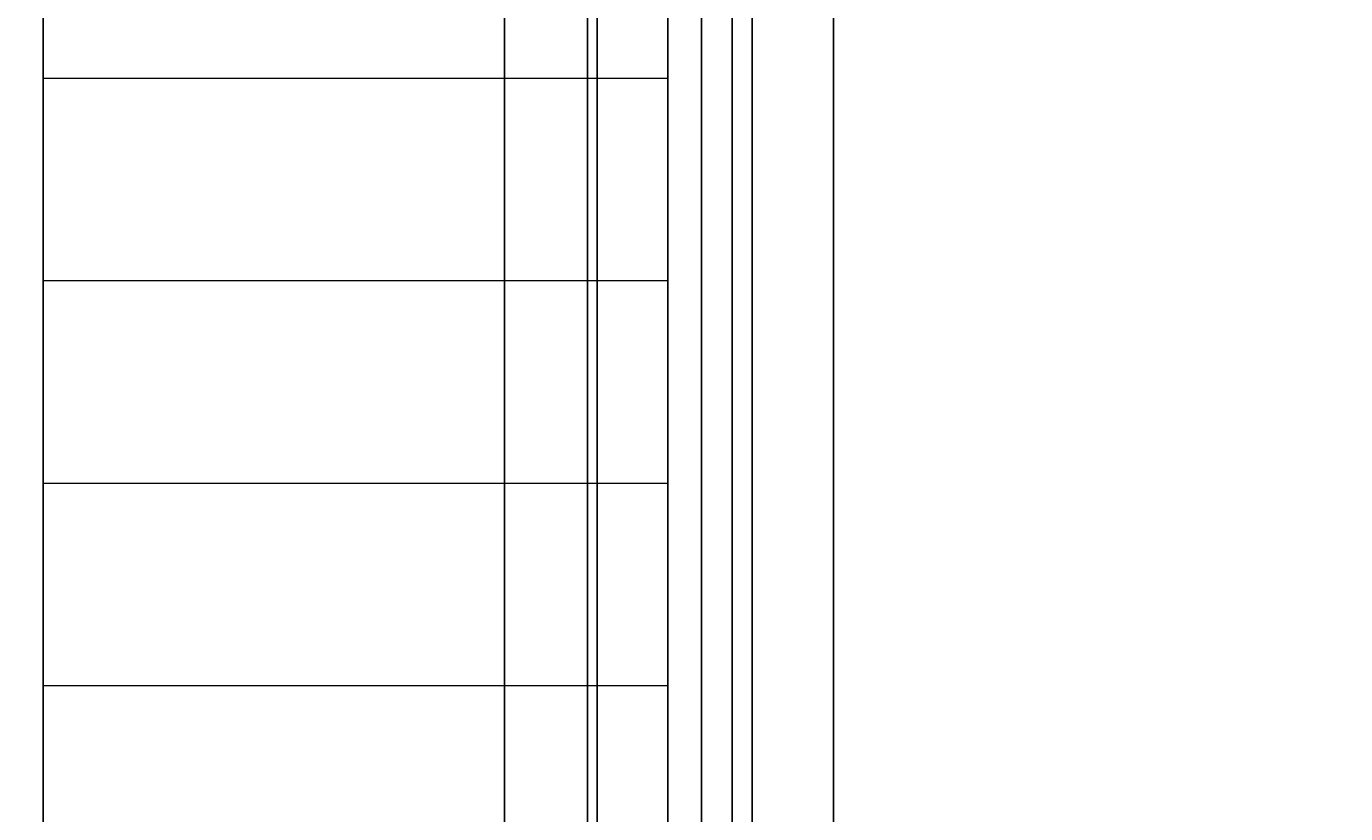
# Model space of a CAD drawing. Units: inches. Extents: x -6 to 289, y -8 to 323.
# Tile 60 of 107: x 147 to 186, y 182 to 206. Entities that reach past the tile are written whole.
import ezdxf

# ---------------------------------------------------------------- set-up
doc = ezdxf.new("R2010")
doc.units = ezdxf.units.IN
doc.header["$MEASUREMENT"] = 0
for name, color, linetype, lineweight in [('A-ANNO-DIMS', 2, 'Continuous', 18), ('A-ELEV-PATT', 8, 'Continuous', 13), ('A-GLAZ', 4, 'Continuous', 25)]:
    doc.layers.add(name, color=color, linetype=linetype, lineweight=lineweight)
doc.styles.get("Standard").update_dxf_attribs({"font": 'arial.ttf'})
doc.dimstyles.get("Standard").update_dxf_attribs({"dimtxt": 0.18, "dimasz": 0.18, "dimexe": 0.18, "dimexo": 0.0625, "dimgap": 0.09, "dimtad": 0, "dimtih": 1, "dimtoh": 1, "dimdec": 4, "dimzin": 0, "dimdsep": 46, "dimtxsty": 'Standard', "dimcen": 0.09, "dimadec": 0, "dimazin": 0, "dimtfac": 1, "dimtdec": 4, "dimtofl": 0, "dimtmove": 0, "dimatfit": 3, "dimfxl": 1, "dimtolj": 1, "dimtzin": 0, "dimarcsym": 0})

# ---------------------------------------------------------------- blocks, each defined once
blk = doc.blocks.new('*U4')
for p, q in [((21, 1.5), (21, 46.5)), ((40.5, 46.5), (40.5, 1.5))]:
    blk.add_line(p, q)
blk.add_lwpolyline([(0, 0), (0, 48), (42, 48), (42, 0)], close=True)
blk.add_lwpolyline([(21, 45.5), (39.5, 45.5), (39.5, 2.5), (21, 2.5)])
blk = doc.blocks.new('*D25')
at = {"layer": 'A-ANNO-DIMS', "color": 0, "lineweight": -2, "transparency": 16777216}
for p, q in [((126.946, 226.654), (288.653, 226.654)), ((288.473, 226.474), (288.473, 202.836)), ((288.473, 178.834), (288.473, 202.472)), ((126.946, 178.654), (288.653, 178.654))]:
    blk.add_line(p, q, dxfattribs=at)
at = {"layer": 'A-ANNO-DIMS', "color": 0, "transparency": 16777216}
for points in [[(288.443, 226.474), (288.503, 226.474), (288.473, 226.654)], [(288.443, 178.834), (288.503, 178.834), (288.473, 178.654)]]:
    blk.add_solid(points, dxfattribs=at)
at = {"layer": 'Defpoints', "color": 0, "transparency": 16777216}
for p in [(126.883, 226.654), (288.473, 226.654), (126.883, 178.654)]:
    blk.add_point(p, dxfattribs=at)
at = {"layer": 'A-ANNO-DIMS', "color": 0, "transparency": 16777216, "insert": (288.473, 202.654), "char_height": 0.18, "attachment_point": 5}
blk.add_mtext('\\A1;48', dxfattribs=at)
blk = doc.blocks.new('*D37')
at = {"layer": 'A-ANNO-DIMS', "color": 0, "lineweight": -2, "transparency": 16777216}
for p, q in [((166.446, 224.154), (288.653, 224.154)), ((288.473, 223.974), (288.473, 202.836)), ((288.473, 181.334), (288.473, 202.472)), ((166.446, 181.154), (288.653, 181.154))]:
    blk.add_line(p, q, dxfattribs=at)
at = {"layer": 'A-ANNO-DIMS', "color": 0, "transparency": 16777216}
for points in [[(288.443, 223.974), (288.503, 223.974), (288.473, 224.154)], [(288.443, 181.334), (288.503, 181.334), (288.473, 181.154)]]:
    blk.add_solid(points, dxfattribs=at)
at = {"layer": 'Defpoints', "color": 0, "transparency": 16777216}
for p in [(166.383, 224.154), (288.473, 224.154), (166.383, 181.154)]:
    blk.add_point(p, dxfattribs=at)
at = {"layer": 'A-ANNO-DIMS', "color": 0, "transparency": 16777216, "insert": (288.473, 202.654), "char_height": 0.18, "attachment_point": 5}
blk.add_mtext('\\A1;43', dxfattribs=at)
blk = doc.blocks.new('*D76')
at = {"layer": 'A-ANNO-DIMS', "color": 0, "lineweight": -2, "transparency": 16777216}
for p, q in [((142.296, 51.148), (142.296, 322.969)), ((164.296, 51.148), (164.296, 322.969)), ((142.476, 322.789), (153.076, 322.789)), ((164.116, 322.789), (153.516, 322.789))]:
    blk.add_line(p, q, dxfattribs=at)
at = {"layer": 'A-ANNO-DIMS', "color": 0, "transparency": 16777216}
for points in [[(142.476, 322.819), (142.476, 322.759), (142.296, 322.789)], [(164.116, 322.819), (164.116, 322.759), (164.296, 322.789)]]:
    blk.add_solid(points, dxfattribs=at)
at = {"layer": 'Defpoints', "color": 0, "transparency": 16777216}
for p in [(164.296, 322.789), (142.296, 51.085), (164.296, 51.085)]:
    blk.add_point(p, dxfattribs=at)
at = {"layer": 'A-ANNO-DIMS', "color": 0, "transparency": 16777216, "insert": (153.296, 322.789), "char_height": 0.18, "attachment_point": 5}
blk.add_mtext('\\A1;22', dxfattribs=at)
blk = doc.blocks.new('*D77')
at = {"layer": 'A-ANNO-DIMS', "color": 0, "lineweight": -2, "transparency": 16777216}
for p, q in [((164.296, 51.148), (164.296, 322.969)), ((168.296, 51.148), (168.296, 322.969)), ((164.476, 322.789), (166.144, 322.789)), ((168.116, 322.789), (166.448, 322.789))]:
    blk.add_line(p, q, dxfattribs=at)
at = {"layer": 'A-ANNO-DIMS', "color": 0, "transparency": 16777216}
for points in [[(164.476, 322.819), (164.476, 322.759), (164.296, 322.789)], [(168.116, 322.819), (168.116, 322.759), (168.296, 322.789)]]:
    blk.add_solid(points, dxfattribs=at)
at = {"layer": 'Defpoints', "color": 0, "transparency": 16777216}
for p in [(168.296, 322.789), (164.296, 51.085), (168.296, 51.085)]:
    blk.add_point(p, dxfattribs=at)
at = {"layer": 'A-ANNO-DIMS', "color": 0, "transparency": 16777216, "insert": (166.296, 322.789), "char_height": 0.18, "attachment_point": 5}
blk.add_mtext('\\A1;4', dxfattribs=at)
blk = doc.blocks.new('*D78')
at = {"layer": 'A-ANNO-DIMS', "color": 0, "lineweight": -2, "transparency": 16777216}
for p, q in [((168.296, 51.148), (168.296, 322.969)), ((171.296, 51.148), (171.296, 322.969)), ((168.476, 322.789), (169.647, 322.789)), ((171.116, 322.789), (169.945, 322.789))]:
    blk.add_line(p, q, dxfattribs=at)
at = {"layer": 'A-ANNO-DIMS', "color": 0, "transparency": 16777216}
for points in [[(168.476, 322.819), (168.476, 322.759), (168.296, 322.789)], [(171.116, 322.819), (171.116, 322.759), (171.296, 322.789)]]:
    blk.add_solid(points, dxfattribs=at)
at = {"layer": 'Defpoints', "color": 0, "transparency": 16777216}
for p in [(171.296, 322.789), (168.296, 51.085), (171.296, 51.085)]:
    blk.add_point(p, dxfattribs=at)
at = {"layer": 'A-ANNO-DIMS', "color": 0, "transparency": 16777216, "insert": (169.796, 322.789), "char_height": 0.18, "attachment_point": 5}
blk.add_mtext('\\A1;3', dxfattribs=at)
blk = doc.blocks.new('*D79')
at = {"layer": 'A-ANNO-DIMS', "color": 0, "lineweight": -2, "transparency": 16777216}
for p, q in [((171.296, 118.033), (171.296, 322.969)), ((188.292, 116.842), (188.292, 322.969)), ((171.476, 322.789), (179.339, 322.789)), ((188.112, 322.789), (180.249, 322.789))]:
    blk.add_line(p, q, dxfattribs=at)
at = {"layer": 'A-ANNO-DIMS', "color": 0, "transparency": 16777216}
for points in [[(171.476, 322.819), (171.476, 322.759), (171.296, 322.789)], [(188.112, 322.819), (188.112, 322.759), (188.292, 322.789)]]:
    blk.add_solid(points, dxfattribs=at)
at = {"layer": 'Defpoints', "color": 0, "transparency": 16777216}
for p in [(188.292, 322.789), (171.296, 117.971), (188.292, 116.779)]:
    blk.add_point(p, dxfattribs=at)
at = {"layer": 'A-ANNO-DIMS', "color": 0, "transparency": 16777216, "insert": (179.794, 322.789), "char_height": 0.18, "attachment_point": 5}
blk.add_mtext('\\A1;16.996', dxfattribs=at)
blk = doc.blocks.new('*D94')
at = {"layer": 'A-ANNO-DIMS', "color": 0, "lineweight": -2, "transparency": 16777216}
for p, q in [((118.164, 159.411), (118.164, 322.969)), ((161.552, 159.411), (161.552, 322.969)), ((118.344, 322.789), (139.46, 322.789)), ((161.372, 322.789), (140.256, 322.789))]:
    blk.add_line(p, q, dxfattribs=at)
at = {"layer": 'A-ANNO-DIMS', "color": 0, "transparency": 16777216}
for points in [[(118.344, 322.819), (118.344, 322.759), (118.164, 322.789)], [(161.372, 322.819), (161.372, 322.759), (161.552, 322.789)]]:
    blk.add_solid(points, dxfattribs=at)
at = {"layer": 'Defpoints', "color": 0, "transparency": 16777216}
for p in [(161.552, 322.789), (118.164, 159.348), (161.552, 159.348)]:
    blk.add_point(p, dxfattribs=at)
at = {"layer": 'A-ANNO-DIMS', "color": 0, "transparency": 16777216, "insert": (139.858, 322.789), "char_height": 0.18, "attachment_point": 5}
blk.add_mtext('\\A1;43.39', dxfattribs=at)
blk = doc.blocks.new('*D95')
at = {"layer": 'A-ANNO-DIMS', "color": 0, "lineweight": -2, "transparency": 16777216}
for p, q in [((161.552, 159.411), (161.552, 322.969)), ((164.004, 159.411), (164.004, 322.969)), ((161.732, 322.789), (162.452, 322.789)), ((163.824, 322.789), (163.104, 322.789))]:
    blk.add_line(p, q, dxfattribs=at)
at = {"layer": 'A-ANNO-DIMS', "color": 0, "transparency": 16777216}
for points in [[(161.732, 322.819), (161.732, 322.759), (161.552, 322.789)], [(163.824, 322.819), (163.824, 322.759), (164.004, 322.789)]]:
    blk.add_solid(points, dxfattribs=at)
at = {"layer": 'Defpoints', "color": 0, "transparency": 16777216}
for p in [(164.004, 322.789), (161.552, 159.348), (164.004, 159.348)]:
    blk.add_point(p, dxfattribs=at)
at = {"layer": 'A-ANNO-DIMS', "color": 0, "transparency": 16777216, "insert": (162.778, 322.789), "char_height": 0.18, "attachment_point": 5}
blk.add_mtext('\\A1;2.45', dxfattribs=at)
blk = doc.blocks.new('*D96')
at = {"layer": 'A-ANNO-DIMS', "color": 0, "lineweight": -2, "transparency": 16777216}
for p, q in [((164.004, 159.411), (164.004, 322.969)), ((200.616, 159.411), (200.616, 322.969)), ((164.184, 322.789), (181.934, 322.789)), ((200.436, 322.789), (182.686, 322.789))]:
    blk.add_line(p, q, dxfattribs=at)
at = {"layer": 'A-ANNO-DIMS', "color": 0, "transparency": 16777216}
for points in [[(164.184, 322.819), (164.184, 322.759), (164.004, 322.789)], [(200.436, 322.819), (200.436, 322.759), (200.616, 322.789)]]:
    blk.add_solid(points, dxfattribs=at)
at = {"layer": 'Defpoints', "color": 0, "transparency": 16777216}
for p in [(200.616, 322.789), (164.004, 159.348), (200.616, 159.348)]:
    blk.add_point(p, dxfattribs=at)
at = {"layer": 'A-ANNO-DIMS', "color": 0, "transparency": 16777216, "insert": (182.31, 322.789), "char_height": 0.18, "attachment_point": 5}
blk.add_mtext('\\A1;36.61', dxfattribs=at)

msp = doc.modelspace()

# ---------------------------------------------------------------- hatches: boundary and pattern name
at = {"layer": 'A-ELEV-PATT'}
h = msp.add_hatch(dxfattribs=at)
h.set_pattern_fill('_USER', color=256, scale=6, pattern_type=0)
h.set_pattern_definition([(0, (0, 0), (0, 6), [])])
h.paths.add_polyline_path([(184.1244, 48.0851), (124.008, 48.0851), (124.008, 10.2888), (184.1244, 10.2888)])
h.paths.add_polyline_path([(244.2408, 48.0851), (186.3604, 48.0851), (186.3604, 10.2888), (244.2408, 10.2888)])
h.paths.add_polyline_path([(208.2918, 114.2795), (190.7918, 114.2795), (190.7918, 71.2795), (208.2918, 71.2795)])
h.paths.add_polyline_path([(227.7918, 114.2795), (209.2918, 114.2795), (209.2918, 71.2795), (227.7918, 71.2795)])
h.paths.add_polyline_path([(211.2918, 224.3887), (190.7918, 224.3887), (190.7918, 162.3484), (211.2918, 162.3484)])
h.paths.add_polyline_path([(233.7918, 224.3887), (212.2918, 224.3887), (212.2918, 162.3484), (233.7918, 162.3484)])
h.paths.add_polyline_path([(166.3835, 224.154), (147.8835, 224.154), (147.8835, 181.154), (166.3835, 181.154)])
h.paths.add_polyline_path([(146.8835, 224.154), (129.3835, 224.154), (129.3835, 181.154), (146.8835, 181.154)])

# ---------------------------------------------------------------- block references
at = {"layer": 'A-GLAZ'}
msp.add_blockref('*U4', (126.8835, 178.654), dxfattribs=at)

# ---------------------------------------------------------------- dimensions: what is measured, and where the dimension line sits
at = {"layer": 'A-ANNO-DIMS'}
for base, p1, p2, override, picture, middle in [((161.5522, 322.7888), (118.1638, 159.3484), (161.5522, 159.3484), {"dimdec": 2, "dimlfac": 1, "dimrnd": 0, "dimzin": 0, "dimdsep": 46, "dimlunit": 2}, '*D94', (139.858, 322.7888)), ((164.296, 322.7888), (142.296, 51.0851), (164.296, 51.0851), {"dimdec": 0, "dimlfac": 1, "dimrnd": 0, "dimzin": 0, "dimdsep": 46, "dimlunit": 2}, '*D76', (153.296, 322.7888)), ((164.0039, 322.7888), (161.5522, 159.3484), (164.0039, 159.3484), {"dimdec": 2, "dimlfac": 1, "dimrnd": 0, "dimzin": 0, "dimdsep": 46, "dimlunit": 2}, '*D95', (162.7781, 322.7888)), ((200.6162, 322.7888), (164.0039, 159.3484), (200.6162, 159.3484), {"dimdec": 2, "dimlfac": 1, "dimrnd": 0, "dimzin": 0, "dimdsep": 46, "dimlunit": 2}, '*D96', (182.3101, 322.7888)), ((168.296, 322.7888), (164.296, 51.0851), (168.296, 51.0851), {"dimdec": 0, "dimlfac": 1, "dimrnd": 0, "dimzin": 0, "dimdsep": 46, "dimlunit": 2}, '*D77', (166.296, 322.7888)), ((171.296, 322.7888), (168.296, 51.0851), (171.296, 51.0851), {"dimdec": 0, "dimlfac": 1, "dimrnd": 0, "dimzin": 0, "dimdsep": 46, "dimlunit": 2}, '*D78', (169.796, 322.7888)), ((188.2918, 322.7888), (171.296, 117.9706), (188.2918, 116.7795), {"dimdec": 3, "dimlfac": 1, "dimrnd": 0, "dimzin": 0, "dimdsep": 46, "dimlunit": 2}, '*D79', (179.7939, 322.7888))]:
    dim = msp.add_linear_dim(base=base, p1=p1, p2=p2, dimstyle='Standard', override=override, dxfattribs=at)
    dim.commit()
    dim.dimension.update_dxf_attribs({"geometry": picture, "text_midpoint": middle})
for base, p1, p2, picture in [((288.4733, 226.654), (126.8835, 178.654), (126.8835, 226.654), '*D25'), ((288.4733, 224.154), (166.3835, 181.154), (166.3835, 224.154), '*D37')]:
    dim = msp.add_linear_dim(base=base, p1=p1, p2=p2, angle=90, dimstyle='Standard', override={"dimdec": 0, "dimlfac": 1, "dimrnd": 0, "dimzin": 0, "dimdsep": 46, "dimlunit": 2}, dxfattribs=at)
    dim.commit()
    dim.dimension.update_dxf_attribs({"geometry": picture, "text_midpoint": (288.4733, 202.654)})

doc.saveas('drawing.dxf')
